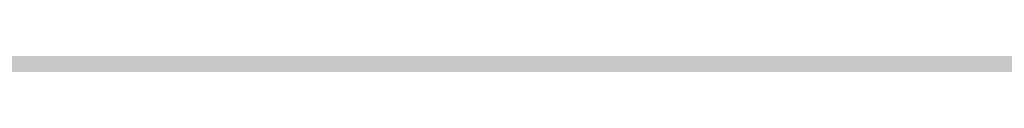
# Model space of a CAD drawing. Units: inches. Extents: x 2091 to 2899, y 967 to 2217.
# Tile 211 of 256: x 2203.2571 to 2203.4104, y 1152.2473 to 1152.2475. Entities that reach past the tile are written whole.
import ezdxf

# ---------------------------------------------------------------- set-up
doc = ezdxf.new("R2010")
doc.units = ezdxf.units.IN
doc.layers.add('A-WALL-PATT', color=141, linetype='Continuous', lineweight=13, true_color=0xadddf7)

msp = doc.modelspace()

# ---------------------------------------------------------------- hatches: boundary and pattern name
at = {"layer": 'A-WALL-PATT'}
h = msp.add_hatch(color=256, dxfattribs=at)
h.dxf.hatch_style = 1
h.paths.add_polyline_path([(2803.1436, 2050.91906), (2203.1436, 2050.91906), (2203.1436, 1090.91906), (2803.1436, 1090.91906)])
h.paths.add_polyline_path([(2635.79885, 1147.54046), (2674.52405, 1147.54046, 0.376086), (2678.52967, 1152.8802), (2678.52967, 1159.55647, 0.333335), (2674.52432, 1163.56185), (2674.52432, 1163.56185), (2674.52432, 1192.93439), (2635.80597, 1192.93439), (2597.08762, 1192.93439), (2597.08762, 1163.56185, 0.333335), (2593.08228, 1159.55647), (2593.08228, 1152.8802, 0.376086), (2597.08789, 1147.54046)], flags=0)
h.paths.add_polyline_path([(2436.01043, 1278.24078, 0.000483), (2435.95264, 1278.21503, -0.001328), (2435.93563, 1278.11169, -0.001711), (2436.11644, 1278.04076, 0.002185)], flags=0)
h.paths.add_polyline_path([(2794.1436, 1143.41906), (2794.1436, 1347.41906), (2543.37017, 1347.41906), (2543.37017, 1351.91906), (2794.1436, 1351.91906), (2794.1436, 1392.71355), (2793.9474, 1392.71355), (2793.9474, 1473.5369), (2794.1436, 1473.5369), (2794.1436, 1531.91906), (2650.1436, 1531.91906), (2650.1436, 1536.41906), (2794.1436, 1536.41906), (2794.1436, 1692.41906), (2609.37561, 1692.41906), (2609.37561, 1644.41906), (2604.87561, 1644.41906), (2604.87561, 1744.91906), (2609.37561, 1744.91906), (2609.37561, 1696.91906), (2794.1436, 1696.91906), (2794.1436, 1780.91906), (2609.6436, 1780.91906), (2493.87561, 1780.91906), (2493.87561, 1785.41906), (2609.6436, 1785.41906), (2794.1436, 1785.41906), (2794.1436, 1847.93882), (2793.95122, 1847.93882), (2793.95122, 1928.76217), (2794.1436, 1928.76217), (2794.1436, 1941.41906), (2614.1436, 1941.41906), (2614.1436, 1821.41906), (2609.6436, 1821.41906), (2609.6436, 1941.41906), (2392.1436, 1941.41906), (2392.1436, 1819.91906), (2387.6436, 1819.91906), (2387.6436, 1941.41906), (2212.1436, 1941.41906), (2212.1436, 1783.91906), (2392.1436, 1783.91906), (2392.1436, 1780.91906), (2212.1436, 1780.91906), (2212.1436, 1629.41906), (2387.6436, 1629.41906), (2387.6436, 1744.91906), (2392.1436, 1744.91906), (2392.1436, 1627.91906), (2317.1436, 1627.91906), (2317.1436, 1551.41906), (2317.1436, 1536.41906), (2459.38359, 1536.41906), (2459.38359, 1602.39648), (2463.88359, 1602.39648), (2463.88359, 1531.91906), (2456.6436, 1531.91906), (2456.6436, 1529.91906), (2452.1436, 1529.91906), (2452.1436, 1531.91906), (2312.6436, 1531.91906), (2312.6436, 1551.41906), (2306.1436, 1551.41906), (2306.1436, 1555.91906), (2308.1436, 1555.91906), (2308.1436, 1551.41906), (2312.6436, 1551.41906), (2312.6436, 1627.91906), (2212.1436, 1627.91906), (2212.1436, 1555.91906), (2270.1436, 1555.91906), (2270.1436, 1551.41906), (2212.1436, 1551.41906), (2212.1436, 1351.91906), (2272.1436, 1351.91906), (2272.1436, 1347.41906), (2212.1436, 1347.41906), (2212.1436, 1275.41906), (2308.1436, 1275.41906), (2308.1436, 1351.91906), (2452.1436, 1351.91906), (2452.1436, 1493.91906), (2456.6436, 1493.91906), (2456.6436, 1347.41906), (2312.6436, 1347.41906), (2312.6436, 1270.91906), (2212.1436, 1270.91906), (2212.1436, 1099.91906), (2281.23752, 1099.91906), (2282.87104, 1110.9138), (2282.00834, 1116.9966), (2278.55774, 1121.4204), (2268.20564, 1128.0562), (2272.08764, 1128.0562), (2273.81294, 1131.927), (2279.42034, 1134.6919), (2285.02784, 1135.2449), (2287.61584, 1137.4568), (2288.04714, 1138.0098), (2289.34114, 1140.7747), (2291.06654, 1139.6687), (2292.36054, 1135.2449), (2295.37984, 1136.9038), (2296.24254, 1135.7979), (2297.10524, 1133.033), (2300.12464, 1138.0098), (2303.14394, 1138.0098), (2304.43794, 1135.7979), (2303.14394, 1133.586), (2306.59464, 1134.6919), (2307.88874, 1133.033), (2310.90804, 1135.2449), (2313.92744, 1134.1389), (2315.62686, 1132.4271), (2308.32004, 1117.5496), (2290.20384, 1109.8079), (2288.90984, 1103.1721), (2289.27231, 1099.91906), (2434.91823, 1099.91906), (2431.59323, 1124.78806), (2429.93023, 1169.55306), (2430.92718, 1240.51969), (2435.65893, 1238.18613), (2437.13523, 1196.55406), (2438.79823, 1143.97306), (2442.67823, 1111.99806), (2446.55823, 1099.91906), (2794.1436, 1099.91906), (2794.1436, 1138.91906), (2548.03245, 1138.91906), (2548.03245, 1143.41906), (2548.03245, 1148.81906), (2546.66846, 1148.03156), (2528.68569, 1179.17862, 0.256256), (2512.03245, 1148.81906), (2512.03245, 1143.41906), (2512.03245, 1138.91906), (2507.53245, 1138.91906), (2507.53245, 1143.41906), (2507.53245, 1148.81906, 0.256256), (2490.8792, 1179.17862), (2472.89644, 1148.03156), (2471.53245, 1148.81906), (2471.53245, 1143.41906), (2467.03245, 1143.41906), (2467.03245, 1269.94579, 0.039061), (2460.90999, 1273.58006), (2467.03245, 1273.58006), (2467.03245, 1286.32536, 0.014511), (2465.21619, 1286.76191), (2467.03245, 1287.05258), (2467.03245, 1323.41906), (2471.53245, 1323.41906), (2471.53245, 1148.81906), (2489.53245, 1179.99597), (2490.89644, 1179.20847), (2490.8792, 1179.17862, -0.256256), (2507.53245, 1148.81906), (2507.53245, 1143.41906), (2512.03245, 1143.41906), (2512.03245, 1148.81906, -0.256256), (2528.68569, 1179.17862), (2528.66846, 1179.20847), (2530.03245, 1179.99597), (2548.03245, 1148.81906), (2548.03245, 1143.41906)], flags=16)
h.paths.add_polyline_path([(2607.76855, 1200.94508), (2607.76855, 1265.03063), (2597.08762, 1281.05201), (2619.78459, 1281.05201), (2627.79528, 1337.12686), (2635.79885, 1337.12686), (2643.81666, 1337.12686), (2651.82736, 1281.05201), (2674.52432, 1281.05201), (2663.8434, 1265.03063), (2663.8434, 1200.94508), (2635.80597, 1200.94508)], flags=0)
edge = h.paths.add_edge_path(flags=0)
edge.add_ellipse((13303.89622, 1272.99872), major_axis=(-10595.31304, 0), ratio=0.84230387009, start_angle=0.628237219, end_angle=0.6465541, ccw=False)
edge.add_ellipse((2711.70045, 1156.85268), major_axis=(2.21977, 0), ratio=0.8423039, start_angle=111.53524, end_angle=180.62824, ccw=False)
edge.add_ellipse((13303.15629, 1272.99872), major_axis=(-10593.02631, 0), ratio=0.84230386954, start_angle=0.528271472, end_angle=0.646554097, ccw=False)
edge.add_line((2710.7646, 1175.3333), (2710.12999, 1175.3333))
edge.add_ellipse((2710.12999, 1176.57978), major_axis=(1.47985, 0), ratio=0.8423039, start_angle=180, end_angle=270, ccw=False)
edge.add_line((2708.65014, 1176.57978), (2708.65014, 1200.78291))
edge.add_ellipse((2710.12999, 1200.78291), major_axis=(1.47985, 0), ratio=0.8423039, start_angle=90, end_angle=180, ccw=False)
edge.add_line((2710.12999, 1202.02939), (2710.46508, 1202.02939))
edge.add_ellipse((13303.15629, 1272.99872), major_axis=(-10593.02631, 0), ratio=0.84230386954, start_angle=-0.090229089, end_angle=0.383866779, ccw=False)
edge.add_ellipse((2710.12999, 1290.92703), major_axis=(-1.47985, 0), ratio=0.8423039, start_angle=0, end_angle=90, ccw=False)
edge.add_line((2708.65014, 1290.92703), (2708.65014, 1315.13017))
edge.add_ellipse((2710.12999, 1315.13017), major_axis=(-1.47985, 0), ratio=0.8423039, start_angle=-90, end_angle=0, ccw=False)
edge.add_line((2710.12999, 1316.37665), (2710.70631, 1316.37665))
edge.add_ellipse((3238.40172, 1296.28957), major_axis=(528.234, 0), ratio=0.84230387, start_angle=176.3495724, end_angle=177.8200497, ccw=False)
edge.add_ellipse((2775.06304, 1071.4507), major_axis=(313.30776, 0), ratio=0.84230387, start_angle=102.1259656, end_angle=103.780529, ccw=False)
edge.add_ellipse((2775.06304, 1078.3057), major_axis=(-305.30289, 0), ratio=0.84230387, start_angle=-79.790461, end_angle=-77.5553727, ccw=False)
edge.add_ellipse((2695.14177, 1541.97538), major_axis=(-250.96022, 0), ratio=0.84230387, start_angle=99.256566, end_angle=102.5549326)
edge.add_line((2741.41033, 1334.21426), (2747.13255, 1337.37848))
edge.add_ellipse((2747.53862, 1336.85748), major_axis=(-0.73992, 0), ratio=0.842304, start_angle=270, end_angle=307.93313, ccw=False)
edge.add_ellipse((2747.53862, 1336.85748), major_axis=(-0.73992, 0), ratio=0.842304, start_angle=232.06687, end_angle=270, ccw=False)
edge.add_line((2747.94469, 1337.37848), (2753.66691, 1334.21426))
edge.add_ellipse((2799.93547, 1541.97538), major_axis=(250.96022, 0), ratio=0.84230387, start_angle=257.4450674, end_angle=260.743434)
edge.add_ellipse((2720.01419, 1078.3057), major_axis=(305.30289, 0), ratio=0.84230387, start_angle=77.5553727, end_angle=79.790461, ccw=False)
edge.add_ellipse((2720.01419, 1071.4507), major_axis=(-313.30776, 0), ratio=0.84230387, start_angle=256.219471, end_angle=257.8740344, ccw=False)
edge.add_ellipse((2256.67551, 1296.28957), major_axis=(-528.234, 0), ratio=0.84230387, start_angle=182.1799503, end_angle=183.6504276, ccw=False)
edge.add_line((2784.37092, 1316.37665), (2784.94725, 1316.37665))
edge.add_ellipse((2784.94725, 1315.13017), major_axis=(1.47985, 0), ratio=0.8423039, start_angle=0, end_angle=90, ccw=False)
edge.add_line((2786.42709, 1315.13017), (2786.42709, 1290.92703))
edge.add_ellipse((2784.94725, 1290.92703), major_axis=(1.47985, 0), ratio=0.8423039, start_angle=270, end_angle=360, ccw=False)
edge.add_ellipse((-7808.07906, 1272.99872), major_axis=(10593.02631, 0), ratio=0.84230386954, start_angle=-0.383866779, end_angle=0.090229089, ccw=False)
edge.add_line((2784.61216, 1202.02939), (2784.94725, 1202.02939))
edge.add_ellipse((2784.94725, 1200.78291), major_axis=(1.47985, 0), ratio=0.8423039, start_angle=0, end_angle=90, ccw=False)
edge.add_line((2786.42709, 1200.78291), (2786.42709, 1176.57978))
edge.add_ellipse((2784.94725, 1176.57978), major_axis=(-1.47985, 0), ratio=0.8423039, start_angle=90, end_angle=180, ccw=False)
edge.add_line((2784.94725, 1175.3333), (2784.31264, 1175.3333))
edge.add_ellipse((-7808.07906, 1272.99872), major_axis=(10593.02631, 0), ratio=0.84230386954, start_angle=-0.618643196, end_angle=-0.528271472, ccw=False)
edge.add_ellipse((2783.37678, 1156.85268), major_axis=(-2.21977, 0), ratio=0.8423039, start_angle=179.37176, end_angle=248.46476, ccw=False)
edge.add_ellipse((-7808.81898, 1272.99872), major_axis=(-10595.31304, 0), ratio=0.84230386576, start_angle=179.353445923, end_angle=179.371762803, ccw=False)
edge.add_ellipse((2780.2973, 1153.50079), major_axis=(-5.24643, 0), ratio=0.8423039, start_angle=90, end_angle=179.35345, ccw=False)
edge.add_line((2780.2973, 1149.08171), (2714.77993, 1149.08171))
edge.add_ellipse((2714.77993, 1153.50079), major_axis=(5.24643, 0), ratio=0.8423039, start_angle=180.64655, end_angle=270, ccw=False)
edge = h.paths.add_edge_path(flags=0)
edge.add_line((2718.18737, 1151.00783), (2718.18737, 1170.47236))
edge.add_ellipse((2721.14706, 1170.47236), major_axis=(-2.95969, 0), ratio=0.8423039, start_angle=-90, end_angle=0, ccw=False)
edge.add_line((2721.14706, 1172.96532), (2773.93017, 1172.96532))
edge.add_ellipse((2773.93017, 1170.47236), major_axis=(-2.95969, 0), ratio=0.8423039, start_angle=180, end_angle=270, ccw=False)
edge.add_line((2776.88987, 1170.47236), (2776.88987, 1151.00783))
edge.add_line((2776.88987, 1151.00783), (2718.18737, 1151.00783))
edge = h.paths.add_edge_path(flags=0)
edge.add_line((2718.18737, 1180.23415), (2718.18737, 1199.05783))
edge.add_ellipse((2747.53862, 1320.39864), major_axis=(147.01792, 0), ratio=0.84230387, start_angle=256.4018653, end_angle=283.5981347)
edge.add_line((2776.88987, 1199.05783), (2776.88987, 1180.23415))
edge.add_ellipse((2747.53862, 1301.57496), major_axis=(147.01792, 0), ratio=0.84230387, start_angle=256.4018653, end_angle=283.5981347, ccw=False)
edge = h.paths.add_edge_path(flags=0)
edge.add_ellipse((13303.15629, 1272.99872), major_axis=(-10591.54646, 0), ratio=0.84230386955, start_angle=0.055594314, end_angle=0.377764194, ccw=False)
edge.add_line((2711.61686, 1262.72171), (2715.66741, 1249.4954))
edge.add_ellipse((6413.89196, 1241.69192), major_axis=(-3698.23616, 0), ratio=0.8423038695, start_angle=-0.12089737, end_angle=0.36407635)
edge.add_line((2715.76104, 1218.19245), (2711.93431, 1203.16736))
edge = h.paths.add_edge_path(flags=0)
edge.add_line((2718.18737, 1251.07457), (2716.00249, 1267.45044))
edge.add_ellipse((2742.15117, 1202.18954), major_axis=(81.77258, 0), ratio=0.84230387, start_angle=94.277421, end_angle=111.8349538, ccw=False)
edge.add_line((2737.00975, 1270.93063), (2758.06748, 1270.93063))
edge.add_ellipse((2752.92606, 1202.18954), major_axis=(81.77258, 0), ratio=0.84230387, start_angle=68.1650462, end_angle=85.722579, ccw=False)
edge.add_line((2779.07475, 1267.45044), (2776.88987, 1251.07457))
edge.add_ellipse((2750.33806, 1187.88536), major_axis=(79.57966, 0), ratio=0.84230387, start_angle=67.2080851, end_angle=85.1299304)
edge.add_line((2756.03466, 1254.74366), (2739.04258, 1254.74366))
edge.add_ellipse((2744.73917, 1187.88536), major_axis=(79.57966, 0), ratio=0.84230387, start_angle=94.8700696, end_angle=112.7919149)
edge = h.paths.add_edge_path(flags=0)
edge.add_line((2783.14293, 1203.16736), (2779.31619, 1218.19245))
edge.add_ellipse((-918.81473, 1241.69192), major_axis=(3698.23616, 0), ratio=0.8423038695, start_angle=-0.36407635, end_angle=0.12089737)
edge.add_line((2779.40983, 1249.4954), (2783.46037, 1262.72171))
edge.add_ellipse((-7808.07906, 1272.99872), major_axis=(-10591.54646, 0), ratio=0.84230386954, start_angle=179.622235806, end_angle=179.944405687, ccw=False)
edge = h.paths.add_edge_path(flags=0)
edge.add_ellipse((2734.20089, 1286.69044), major_axis=(-0.35661, 6.34008), ratio=0.6038336, start_angle=89.002014, end_angle=253.657408, ccw=False)
edge.add_line((2730.369, 1286.54181), (2730.369, 1301.35198))
edge.add_line((2730.369, 1301.35198), (2735.91331, 1305.2148))
edge.add_ellipse((2736.38492, 1304.73456), major_axis=(0.73992, 0), ratio=0.842304, start_angle=90, end_angle=134.48021, ccw=False)
edge.add_line((2736.38492, 1305.3578), (2738.03278, 1305.3578))
edge.add_line((2738.03278, 1305.3578), (2738.03278, 1307.70793))
edge.add_ellipse((2794.20164, 1307.70793), major_axis=(56.16886, 0), ratio=0.84230387, start_angle=150.56143, end_angle=180, ccw=False)
edge.add_ellipse((2700.87559, 1307.70793), major_axis=(-56.16886, 0), ratio=0.84230387, start_angle=180, end_angle=209.43857, ccw=False)
edge.add_line((2757.04445, 1307.70793), (2757.04445, 1305.3578))
edge.add_line((2757.04445, 1305.3578), (2758.69232, 1305.3578))
edge.add_ellipse((2758.69232, 1304.73456), major_axis=(-0.73992, 0), ratio=0.842304, start_angle=225.51979, end_angle=270, ccw=False)
edge.add_line((2759.16392, 1305.2148), (2764.70823, 1301.35198))
edge.add_line((2764.70823, 1301.35198), (2764.70823, 1286.54181))
edge.add_ellipse((2760.87634, 1286.69044), major_axis=(0.35661, 6.34008), ratio=0.6038336, start_angle=106.342592, end_angle=270.997986, ccw=False)
edge.add_line((2757.04445, 1285.79709), (2757.04445, 1307.70793))
edge.add_ellipse((2700.87559, 1307.70793), major_axis=(-56.16886, 0), ratio=0.84230387, start_angle=180, end_angle=209.43857)
edge.add_ellipse((2794.20164, 1307.70793), major_axis=(56.16886, 0), ratio=0.84230387, start_angle=150.56143, end_angle=180)
edge.add_line((2738.03278, 1307.70793), (2738.03278, 1285.79709))
h.paths.add_polyline_path([(2417.81227, 1104.4497), (2413.49227, 1102.5297), (2410.61227, 1103.9697), (2409.17227, 1106.3697), (2407.25227, 1107.3297), (2406.29227, 1109.7297), (2405.33227, 1114.0497), (2405.33227, 1117.8897), (2406.29227, 1120.1297), (2407.25227, 1119.8097), (2408.84832, 1118.32766), (2410.17395, 1119.42417), (2410.21127, 1120.4057), (2411.04073, 1121.41905), (2410.69927, 1119.8587), (2410.17395, 1119.42417), (2410.08845, 1117.17611), (2411.13284, 1116.20632), (2413.97227, 1119.3297), (2416.85227, 1120.7697), (2416.86972, 1120.79878), (2417.03507, 1119.40512), (2417.89621, 1118.14338), (2418.29227, 1118.3697), (2419.54445, 1120.03927), (2419.36092, 1118.38749), (2419.03211, 1119.35615), (2418.39894, 1118.51193), (2419.25227, 1114.5297), (2418.79409, 1107.19879)], flags=0)
h.paths.add_polyline_path([(2508.87017, 1347.41906), (2508.37017, 1347.41906), (2508.37017, 1351.91906), (2508.87017, 1351.91906)], flags=0)
h.paths.add_polyline_path([(2473.37017, 1347.41906), (2472.37017, 1347.41906), (2467.87017, 1347.41906), (2467.87017, 1455.41906), (2472.37017, 1455.41906), (2472.37017, 1352.41906), (2473.37017, 1352.41906)], flags=0)
h.paths.add_polyline_path([(2352.10624, 1217.4462), (2349.22624, 1218.8862), (2347.78624, 1221.2862), (2345.86624, 1222.2462), (2344.90624, 1224.6462), (2343.94624, 1228.9662), (2343.94624, 1232.8062), (2344.90624, 1235.0462), (2345.86624, 1234.7262), (2347.46229, 1233.24415), (2348.78792, 1234.34066), (2348.82524, 1235.3222), (2349.6547, 1236.33555), (2349.31324, 1234.7752), (2348.78792, 1234.34066), (2348.70242, 1232.0926), (2349.74681, 1231.12282), (2352.58624, 1234.2462), (2355.46624, 1235.6862), (2355.48369, 1235.71528), (2355.64904, 1234.32161), (2356.51018, 1233.05988), (2356.90624, 1233.2862), (2358.15842, 1234.95576), (2357.97489, 1233.30398), (2357.64608, 1234.27264), (2357.01291, 1233.42842), (2357.86624, 1229.4462), (2357.40806, 1222.11529), (2356.42624, 1219.3662)], flags=0)
h.paths.add_polyline_path([(2348.2968, 1112.22442), (2347.0138, 1112.31042), (2345.5298, 1114.12742), (2345.7318, 1115.85842), (2346.8118, 1116.98242), (2346.8118, 1114.64642), (2345.8668, 1114.21442), (2346.8798, 1114.30042)], flags=0)
h.paths.add_polyline_path([(2347.0138, 1110.92642), (2346.2718, 1110.49342), (2346.6098, 1111.18642)], flags=0)
h.paths.add_polyline_path([(2345.8668, 1118.19442), (2345.5298, 1117.32942), (2343.7078, 1118.02142), (2344.3828, 1118.62642)], flags=0)
h.paths.add_polyline_path([(2346.6768, 1109.28242), (2346.0698, 1108.07142), (2345.8668, 1110.06142)], flags=0)
h.paths.add_polyline_path([(2345.0568, 1119.75142), (2343.6398, 1119.75142), (2343.9778, 1121.13542)], flags=0)
h.paths.add_polyline_path([(2345.2598, 1116.55042), (2345.1248, 1115.85842), (2344.9218, 1115.68542), (2344.7198, 1116.37742)], flags=0)
h.paths.add_polyline_path([(2345.6648, 1112.31042), (2345.4618, 1111.53242), (2344.0448, 1111.96442), (2344.6518, 1112.57042)], flags=0)
h.paths.add_polyline_path([(2345.1918, 1113.34942), (2344.4498, 1113.86842), (2344.7198, 1114.38742)], flags=0)
h.paths.add_polyline_path([(2344.6518, 1116.80942), (2344.1798, 1115.68542), (2344.6518, 1115.33942), (2343.9098, 1114.90642), (2343.0328, 1115.94442), (2343.6398, 1116.46342)], flags=0)
h.paths.add_polyline_path([(2345.8668, 1106.68642), (2344.9898, 1105.56242), (2344.5168, 1106.60042)], flags=0)
h.paths.add_polyline_path([(2344.8548, 1110.06142), (2344.5168, 1109.28242), (2344.1128, 1109.71542)], flags=0)
h.paths.add_polyline_path([(2344.0448, 1113.52242), (2343.4378, 1113.08942), (2342.7628, 1113.95442)], flags=0)
h.paths.add_polyline_path([(2344.3148, 1111.01242), (2342.9648, 1110.32042), (2342.9648, 1111.09942)], flags=0)
h.paths.add_polyline_path([(2345.1248, 1104.69742), (2344.5848, 1103.74542), (2344.4498, 1104.26442)], flags=0)
h.paths.add_polyline_path([(2342.8298, 1121.22242), (2341.7498, 1120.53042), (2340.5358, 1121.04942), (2340.1308, 1121.82842), (2340.6708, 1122.95242), (2341.1428, 1121.82842), (2341.6148, 1122.00142)], flags=0)
h.paths.add_polyline_path([(2342.9648, 1119.75142), (2343.0328, 1118.45342), (2342.0878, 1118.02142), (2342.0198, 1119.49142)], flags=0)
h.paths.add_polyline_path([(2342.6948, 1116.89642), (2341.9528, 1116.63642), (2342.0198, 1117.32942)], flags=0)
h.paths.add_polyline_path([(2343.0328, 1112.22442), (2342.0198, 1111.79142), (2341.5478, 1112.22442), (2342.3578, 1113.34942)], flags=0)
h.paths.add_polyline_path([(2343.7748, 1104.43742), (2342.6278, 1102.88042), (2342.6948, 1104.61042), (2343.4378, 1105.12942)], flags=0)
h.paths.add_polyline_path([(2342.0198, 1115.07942), (2340.8058, 1115.51242), (2340.9408, 1116.37742)], flags=0)
h.paths.add_polyline_path([(2341.4808, 1120.09742), (2341.4808, 1119.40542), (2341.0758, 1119.57842), (2341.1428, 1120.09742)], flags=0)
h.paths.add_polyline_path([(2341.8178, 1114.47342), (2340.9408, 1113.08942), (2340.8058, 1114.56042)], flags=0)
h.paths.add_polyline_path([(2341.1428, 1118.54042), (2340.9408, 1116.98242), (2339.0508, 1117.67542), (2339.0508, 1118.62642)], flags=0)
h.paths.add_polyline_path([(2342.6948, 1101.66842), (2341.9528, 1101.84142), (2342.5598, 1102.36142)], flags=0)
h.paths.add_polyline_path([(2340.3328, 1119.66542), (2338.4438, 1119.57842), (2337.9038, 1120.35742), (2339.6578, 1120.61642)], flags=0)
h.paths.add_polyline_path([(2340.3328, 1115.33942), (2340.0628, 1113.69542), (2339.3878, 1115.33942)], flags=0)
h.paths.add_polyline_path([(2341.8178, 1103.83142), (2341.5478, 1102.88042), (2341.1428, 1103.65842)], flags=0)
h.paths.add_polyline_path([(2339.0508, 1122.86642), (2337.2958, 1121.82842), (2337.0938, 1123.12542), (2337.7688, 1123.81842)], flags=0)
h.paths.add_polyline_path([(2339.1178, 1121.74142), (2338.8478, 1121.22242), (2338.1738, 1121.04942), (2338.3758, 1121.56842)], flags=0)
h.paths.add_polyline_path([(2339.1858, 1119.31942), (2338.6458, 1118.71342), (2338.2408, 1118.10742), (2338.2408, 1118.88642)], flags=0)
h.paths.add_polyline_path([(2341.1428, 1101.92842), (2340.6028, 1101.23642), (2340.0628, 1101.84142), (2340.6028, 1102.36142)], flags=0)
h.paths.add_polyline_path([(2337.6338, 1117.76142), (2336.6208, 1118.28042), (2337.2958, 1118.97242)], flags=0)
h.paths.add_polyline_path([(2336.8238, 1119.57842), (2334.7988, 1118.97242), (2335.2038, 1120.35742), (2336.5538, 1120.87642)], flags=0)
h.paths.add_polyline_path([(2339.1178, 1100.45742), (2337.3638, 1100.54342), (2336.7558, 1101.23642)], flags=0)
h.paths.add_polyline_path([(2336.3508, 1122.43342), (2336.0138, 1121.91442), (2334.9338, 1122.43342), (2334.5288, 1123.47142), (2335.7438, 1122.77942)], flags=0)
h.paths.add_polyline_path([(2334.7318, 1120.87642), (2334.2588, 1120.35742), (2334.0568, 1120.78942), (2334.5968, 1121.30842)], flags=0)
h.paths.add_polyline_path([(2334.4618, 1122.17442), (2332.5718, 1121.30842), (2331.3568, 1122.17442), (2332.0998, 1122.86642)], flags=0)
h.paths.add_polyline_path([(2334.2588, 1118.54042), (2333.3818, 1118.45342), (2333.6518, 1119.31942)], flags=0)
h.paths.add_polyline_path([(2335.5418, 1102.27442), (2334.1918, 1102.62042), (2335.2718, 1103.31242)], flags=0)
h.paths.add_polyline_path([(2332.7068, 1119.66542), (2331.6948, 1120.44342), (2332.5048, 1120.78942)], flags=0)
h.paths.add_polyline_path([(2334.7318, 1101.14942), (2333.5168, 1101.58242), (2333.9888, 1101.75542)], flags=0)
h.paths.add_polyline_path([(2332.6398, 1116.63642), (2331.0868, 1116.29042), (2331.9648, 1118.19442)], flags=0)
h.paths.add_polyline_path([(2330.7498, 1121.56842), (2330.2768, 1120.27042), (2328.5228, 1119.31942), (2328.9948, 1121.04942)], flags=0)
h.paths.add_polyline_path([(2330.7498, 1118.62642), (2330.0078, 1117.50242), (2329.8728, 1118.02142)], flags=0)
h.paths.add_polyline_path([(2332.0998, 1102.36142), (2330.5468, 1102.01442), (2331.6948, 1102.96642)], flags=0)
h.paths.add_polyline_path([(2329.5348, 1113.60842), (2329.0628, 1112.31042), (2328.5898, 1113.34942)], flags=0)
h.paths.add_polyline_path([(2328.3878, 1117.84842), (2327.5098, 1116.55042), (2327.1728, 1117.76142)], flags=0)
h.paths.add_polyline_path([(2329.7378, 1106.51342), (2329.5348, 1105.30242), (2328.2528, 1106.08142)], flags=0)
h.paths.add_polyline_path([(2328.6578, 1114.38742), (2328.0498, 1114.12742), (2328.3198, 1114.90642)], flags=0)
h.paths.add_polyline_path([(2328.3198, 1112.22442), (2327.1058, 1112.13742), (2326.7008, 1112.65642)], flags=0)
h.paths.add_polyline_path([(2326.9028, 1115.25242), (2326.7008, 1114.12742), (2325.2158, 1113.60842), (2326.0928, 1115.33942)], flags=0)
h.paths.add_polyline_path([(2326.6328, 1108.33042), (2326.0928, 1107.37942), (2325.8908, 1108.50342), (2326.4978, 1109.10942)], flags=0)
h.paths.add_polyline_path([(2615.1436, 1531.91906), (2609.6436, 1531.91906), (2609.6436, 1620.41906), (2614.1436, 1620.41906), (2614.1436, 1536.41906), (2615.1436, 1536.41906)], flags=0)
h.paths.add_polyline_path([(2545.1436, 1563.41906), (2464.1436, 1563.41906), (2464.1436, 1632.41906), (2509.1436, 1632.41906), (2509.1436, 1627.91906), (2509.1436, 1603.91906), (2468.6436, 1603.91906), (2468.6436, 1567.91906), (2540.6436, 1567.91906), (2540.6436, 1591.91906), (2545.1436, 1591.91906)], flags=0)
h.paths.add_polyline_path([(2388.96905, 1549.98573), (2357.43418, 1549.98573), (2357.43418, 1623.36078), (2399.36278, 1623.36078), (2435.68947, 1623.36078), (2435.59255, 1602.55927), (2435.59255, 1602.39648), (2388.96905, 1602.39648)], flags=0)
h.paths.add_polyline_path([(2388.88063, 1555.80915), (2374.90443, 1555.80915), (2374.90443, 1600.57156), (2374.90443, 1615.45765), (2406.35088, 1615.45765), (2406.35088, 1618.93943), (2412.17429, 1615.45765), (2406.35088, 1611.97586), (2406.35088, 1615.45765), (2388.88063, 1615.45765)], flags=0)
h.paths.add_polyline_path([(2568.87561, 1644.41906), (2453.37561, 1644.41906), (2453.37561, 1785.41906), (2457.87561, 1785.41906), (2457.87561, 1648.91906), (2568.87561, 1648.91906)], flags=0)
h.paths.add_polyline_path([(2212.1436, 1945.91906), (2212.1436, 2041.91906), (2794.1436, 2041.91906), (2794.1436, 1945.91906)], flags=16)
h.paths.add_polyline_path([(2271.08273, 1964.31724), (2776.85297, 1964.31724), (2776.85297, 2037.16962), (2271.08273, 2037.16962)], flags=8)
h.paths.add_polyline_path([(2380.64929, 1536.82414), (2461.04081, 1536.82414), (2461.04081, 1554.65259), (2380.64929, 1554.65259)], flags=8)
h.paths.add_polyline_path([(2240.75571, 1609.72545), (2309.18583, 1609.72545), (2309.18583, 1617.6982), (2240.75571, 1617.6982)], flags=8)
h.paths.add_polyline_path([(2212.67726, 1313.5041), (2282.59152, 1313.5041), (2282.59152, 1322.74524), (2212.67726, 1322.74524)], flags=8)
h.paths.add_polyline_path([(2457.11198, 1114.77857), (2558.48158, 1114.77857), (2558.48158, 1142.21968), (2457.11198, 1142.21968)], flags=8)
h.paths.add_polyline_path([(2473.44234, 1273.01007), (2604.64123, 1273.01007), (2604.64123, 1318.34693), (2473.44234, 1318.34693)], flags=8)
h.paths.add_polyline_path([(2638.8763, 1626.97743), (2684.25037, 1627.97674), (2684.03848, 1637.59749), (2638.66442, 1636.59819)], flags=8)
h.paths.add_polyline_path([(2537.59055, 1453.79345), (2628.38955, 1453.79345), (2628.38955, 1475.34481), (2537.59055, 1475.34481)], flags=8)
h.paths.add_polyline_path([(2504.13764, 1714.6324), (2554.64719, 1714.6324), (2554.64719, 1730.23771), (2504.13764, 1730.23771)], flags=8)
h.paths.add_polyline_path([(2487.50118, 1575.65187), (2535.09712, 1575.65187), (2535.09712, 1598.37765), (2487.50118, 1598.37765)], flags=8)
h.paths.add_polyline_path([(2709.0994, 1735.71028), (2740.0166, 1735.71028), (2740.0166, 1749.93764), (2709.0994, 1749.93764)], flags=8)
h.paths.add_polyline_path([(2442.43842, 1792.17166), (2564.72884, 1792.17166), (2564.72884, 1842.00016), (2442.43842, 1842.00016)], flags=8)
h.paths.add_polyline_path([(2655.8158, 1809.64408), (2789.52014, 1806.6938), (2790.08498, 1832.29164), (2656.38064, 1835.24192)], flags=8)
h.paths.add_polyline_path([(2234.8427, 1797.72014), (2368.59285, 1794.76885), (2369.16072, 1820.50413), (2235.41056, 1823.45542)], flags=8)
h.paths.add_polyline_path([(2245.13847, 1644.00633), (2398.42773, 1640.6239), (2398.99484, 1666.32482), (2245.70557, 1669.70725)], flags=8)
h.paths.add_polyline_path([(2306.14285, 1431.16852), (2413.76831, 1428.79369), (2414.33315, 1454.39153), (2306.70768, 1456.76636)], flags=8)
h.paths.add_polyline_path([(2306.83458, 1458.23314), (2393.38048, 1456.32345), (2393.93281, 1481.35436), (2307.38691, 1483.26405)], flags=8)

doc.saveas('drawing.dxf')
